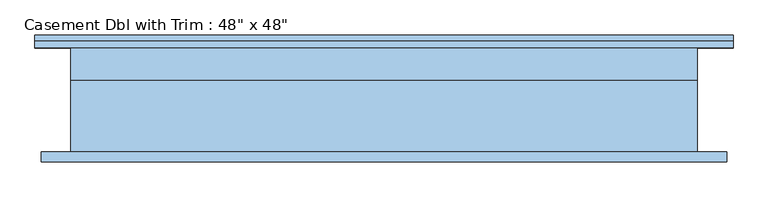
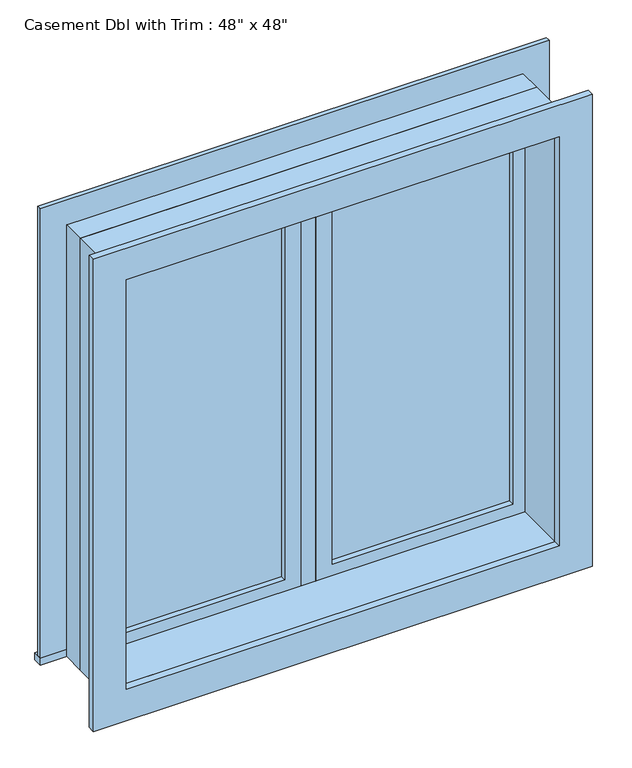
"""IFC4 building model written with IfcOpenShell, lengths in millimetres: window geometry."""

from ifc_helpers import new_model, si_unit, frame, origin, place, context, project, spatial, polyline, outline, extrude, source, transform, mapped, element, save


def window_0862ab64(model_context):
    return source(origin(), model_context, "Body", "SweptSolid", [
        extrude(outline(polyline([(63.5, 85.725), (546.1, 85.725), (546.1, 73.025), (63.5, 73.025), (63.5, 85.725)])), frame((0.0, 0.0, 977.9), z_axis=(0.0, 0.0, 1.0), x_axis=(1.0, 0.0, 0.0)), (0.0, 0.0, 1.0), 1092.2),
        extrude(outline(polyline([(2114.55, 19.05), (933.45, 19.05), (933.45, 590.55), (2114.55, 590.55), (2114.55, 19.05)]), holes=[polyline([(2070.1, 63.5), (2070.1, 546.1), (977.9, 546.1), (977.9, 63.5), (2070.1, 63.5)])]), frame((0.0, 57.15, 0.0), z_axis=(0.0, 1.0, 0.0), x_axis=(0.0, 0.0, 1.0)), (0.0, 0.0, 1.0), 44.45),
        extrude(outline(polyline([(19.05, 57.15), (-19.05, 57.15), (-19.05, 120.65), (19.05, 120.65), (19.05, 57.15)])), frame((0.0, 0.0, 933.45), z_axis=(0.0, 0.0, 1.0), x_axis=(1.0, 0.0, 0.0)), (0.0, 0.0, 1.0), 1181.1),
        extrude(outline(polyline([(-679.45, 146.05), (679.45, 146.05), (679.45, 120.65), (-679.45, 120.65), (-679.45, 146.05)])), frame((0.0, 0.0, 914.4), z_axis=(0.0, 0.0, 1.0), x_axis=(1.0, 0.0, 0.0)), (0.0, 0.0, 1.0), 19.05),
        extrude(outline(polyline([(2114.55, -590.55), (2114.55, 590.55), (933.45, 590.55), (933.45, 679.45), (2203.45, 679.45), (2203.45, -679.45), (933.45, -679.45), (933.45, -590.55), (2114.55, -590.55)])), frame((0.0, 120.65, 0.0), z_axis=(0.0, 1.0, 0.0), x_axis=(0.0, 0.0, 1.0)), (0.0, 0.0, 1.0), 12.7),
        extrude(outline(polyline([(2190.75, 666.75), (2190.75, -666.75), (857.25, -666.75), (857.25, 666.75), (2190.75, 666.75)]), holes=[polyline([(2101.85, 577.85), (946.15, 577.85), (946.15, -577.85), (2101.85, -577.85), (2101.85, 577.85)])]), frame((0.0, -101.6, 0.0), z_axis=(0.0, 1.0, 0.0), x_axis=(0.0, 0.0, 1.0)), (0.0, 0.0, 1.0), 19.05),
        extrude(outline(polyline([(-63.5, 73.025), (-546.1, 73.025), (-546.1, 85.725), (-63.5, 85.725), (-63.5, 73.025)])), frame((0.0, 0.0, 977.9), z_axis=(0.0, 0.0, 1.0), x_axis=(1.0, 0.0, 0.0)), (0.0, 0.0, 1.0), 1092.2),
        extrude(outline(polyline([(2114.55, -590.55), (933.45, -590.55), (933.45, -19.05), (2114.55, -19.05), (2114.55, -590.55)]), holes=[polyline([(2070.1, -546.1), (2070.1, -63.5), (977.9, -63.5), (977.9, -546.1), (2070.1, -546.1)])]), frame((0.0, 57.15, 0.0), z_axis=(0.0, 1.0, 0.0), x_axis=(0.0, 0.0, 1.0)), (0.0, 0.0, 1.0), 44.45),
        extrude(outline(polyline([(2133.6, -609.6), (914.4, -609.6), (914.4, 609.6), (2133.6, 609.6), (2133.6, -609.6)]), holes=[polyline([(2101.85, -577.85), (2101.85, 577.85), (946.15, 577.85), (946.15, -577.85), (2101.85, -577.85)])]), frame((0.0, -82.55, 0.0), z_axis=(0.0, 1.0, 0.0), x_axis=(0.0, 0.0, 1.0)), (0.0, 0.0, 1.0), 139.7),
        extrude(outline(polyline([(2133.6, 609.6), (2133.6, -609.6), (914.4, -609.6), (914.4, 609.6), (2133.6, 609.6)]), holes=[polyline([(2114.55, 590.55), (933.45, 590.55), (933.45, -590.55), (2114.55, -590.55), (2114.55, 590.55)])]), frame((0.0, 57.15, 0.0), z_axis=(0.0, 1.0, 0.0), x_axis=(0.0, 0.0, 1.0)), (0.0, 0.0, 1.0), 63.5),
    ])


if __name__ == "__main__":
    model = new_model("IFC4")
    model_context = context("Model", 3, world=origin())
    ifc_project = project(units=[si_unit("LENGTHUNIT", "METRE", prefix="MILLI")], contexts=[model_context])
    site = spatial("IfcSite", under=ifc_project)
    building = spatial("IfcBuilding", under=site)
    placement = place(None, origin())
    window_shape = window_0862ab64(model_context)
    element("IfcWindow", 1, ObjectType="Casement Dbl with Trim : 48\" x 48\"", at=placement, inside=building, context=model_context, shape_type="MappedRepresentation", body=[
        mapped(window_shape, transform((0.0, 0.0, 0.0), x_axis=(1.0, 0.0, 0.0), y_axis=(0.0, 1.0, 0.0), z_axis=(0.0, 0.0, 1.0))),
    ])
    save(model, "model.ifc")

# Revit data of these elements
# Type "Casement Dbl with Trim : 48\" x 48\""
#   Type Mark = "13"
#   Construction Type Id = "GSP4R"
#   Assembly Code = "B2020100"
#   Analytic Construction = "1/8 in Pilkington single glazing"
#   Visual Light Transmittance = 0.9
#   Solar Heat Gain Coefficient = 0.78
#   Heat Transfer Coefficient (U) = 0.6496 BTU/(h·ft²·°F)
#   Height = 4' - 0"
#   Default Sill Height = 3' - 0"
#   Trim Projection - Ext. = 0' - 0 1/2"
#   Trim Projection - Int. = 0' - 0 3/4"
#   Trim Width - Exterior = 0' - 3 1/2"
#   Trim Width - Interior = 0' - 3 1/2"
#   Width = 4' - 0"
#   Window Inset = 0' - 0 3/4"
#   Define Thermal Properties by = 1
#   Glass Pane Material = Glass
#   Sash Material = Sash
#   Trim Exterior Material = Trim
#   Trim Interior Material = Trim
#   Wall Closure = (empty or 0)
# Element 1 (IfcWindow, "Casement Dbl with Trim : 48\" x 48\"")
#   Materials on its faces: "Sash", "Trim", "Glass"
# Materials
#   "Glass": class "Glass", colour RGB 0 128 192, transparency 0.75, Description = "Soda Lime Glass", Cost = 0
#   "Sash": class "Wood", colour RGB 224 178 126, transparency 0
#   "Trim": class "Wood", colour RGB 224 178 126, transparency 0
